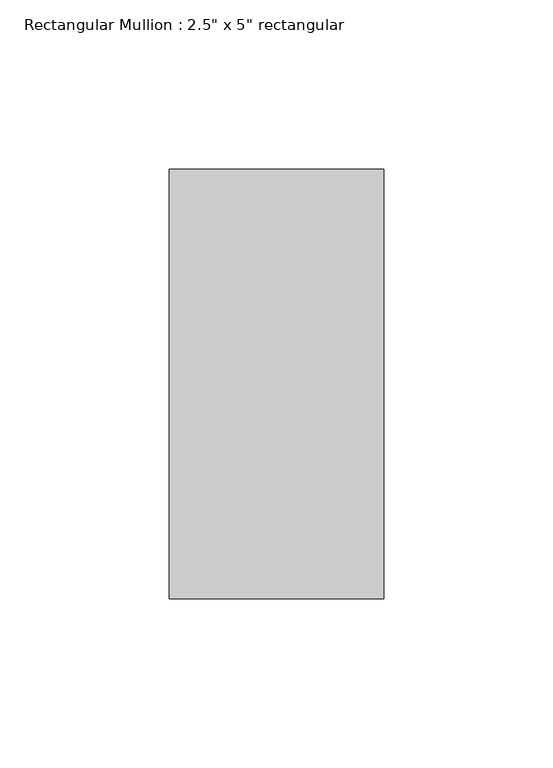
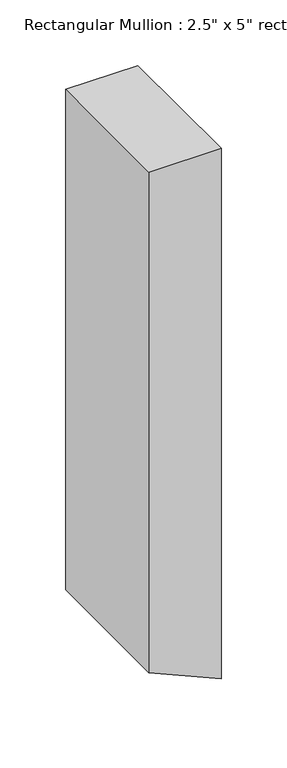
"""IFC4 building model written with IfcOpenShell, lengths in millimetres: member geometry."""

from ifc_helpers import new_model, si_unit, frame, origin, place, context, project, spatial, polyline, outline, extrude, source, transform, mapped, element, save


def member_9b69c4fe(model_context):
    return source(origin(), model_context, "Body", "SweptSolid", [
        extrude(outline(polyline([(0.0, 0.0), (0.0, -63.5), (-465.8044798, -63.5), (-493.4150656, 0.0), (0.0, 0.0)])), frame((0.0, -63.5, 0.0), z_axis=(0.0, 1.0, 0.0), x_axis=(0.0, 0.0, 1.0)), (0.0, 0.0, 1.0), 127.0),
    ])


if __name__ == "__main__":
    model = new_model("IFC4")
    model_context = context("Model", 3, world=origin())
    ifc_project = project(units=[si_unit("LENGTHUNIT", "METRE", prefix="MILLI")], contexts=[model_context])
    site = spatial("IfcSite", under=ifc_project)
    building = spatial("IfcBuilding", under=site)
    placement = place(None, origin())
    member_shape = member_9b69c4fe(model_context)
    element("IfcMember", 1, ObjectType="Rectangular Mullion : 2.5\" x 5\" rectangular", at=placement, inside=building, context=model_context, shape_type="MappedRepresentation", body=[
        mapped(member_shape, transform((0.0, 0.0, 0.0), x_axis=(1.0, 0.0, 0.0), y_axis=(0.0, 1.0, 0.0), z_axis=(0.0, 0.0, 1.0))),
    ])
    save(model, "model.ifc")

# Revit data of these elements
# Type "Rectangular Mullion : 2.5\" x 5\" rectangular"
#   built-in parameter 1007304 = 0.416667 (stored number, unit not read)
#   built-in parameter 1007301 = 0.104167 (stored number, unit not read)
#   built-in parameter 1007300 = 0.104167 (stored number, unit not read)
# Element 1 (IfcMember, "Rectangular Mullion : 2.5\" x 5\" rectangular")
#   Materials on its faces: "door colour"
# Materials
#   "door colour": class "Generic", colour RGB 120 120 120, transparency 0, Cost = 0
